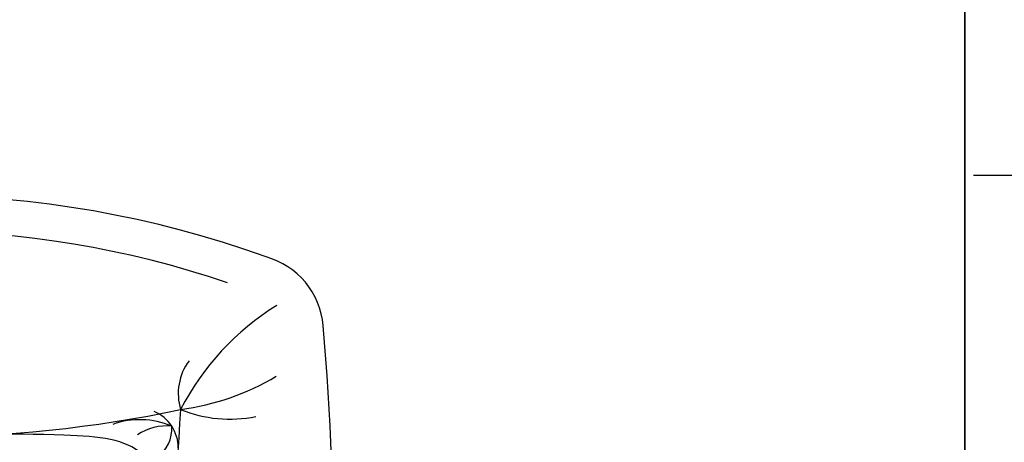
# Model space of a CAD drawing. Units: inches. Extents: x 844 to 2234, y 346 to 1084.
# Tile 88 of 93: x 2010.87 to 2030.9, y 728.83 to 737.43. Entities that reach past the tile are written whole.
import ezdxf

# ---------------------------------------------------------------- set-up
doc = ezdxf.new("R2010")
doc.units = ezdxf.units.IN
doc.header["$MEASUREMENT"] = 0
for name, color, linetype, lineweight in [('A-ANNO-DIMS', 2, 'Continuous', 18), ('A-WALL', 7, 'Continuous', 35), ('furniture', 8, 'Continuous', 18)]:
    doc.layers.add(name, color=color, linetype=linetype, lineweight=lineweight)
doc.layers.add('RA-AP-01$0$FURN', color=3, linetype='Continuous')
doc.layers.add('RA-AP-01$0$WOOD', color=64, linetype='Continuous')
doc.styles.get("Standard").update_dxf_attribs({"font": 'arial.ttf'})
doc.dimstyles.get("Standard").update_dxf_attribs({"dimtxt": 6, "dimasz": 3, "dimexe": 0.18, "dimexo": 0.0625, "dimgap": 0.09, "dimtad": 0, "dimtih": 1, "dimtoh": 1, "dimdec": 1, "dimzin": 0, "dimdsep": 46, "dimlunit": 3, "dimtxsty": 'Standard', "dimblk": 'ARCHTICK', "dimcen": 0.09, "dimadec": 0, "dimazin": 0, "dimtfac": 1, "dimtdec": 1, "dimtofl": 0, "dimtmove": 0, "dimatfit": 3, "dimfxl": 1, "dimtolj": 1, "dimtzin": 0, "dimarcsym": 0})

# ---------------------------------------------------------------- blocks, each defined once
blk = doc.blocks.new('A$C7F4351E2')
at = {"layer": 'RA-AP-01$0$FURN'}
for p, q in [((8.352559572600457, -8.263941955512525), (8.35255957259913, -8.282283310927069)), ((8.352559572600457, -8.927748273106442), (8.35255957259913, -8.909406917691898))]:
    blk.add_line(p, q, dxfattribs=at)
at = {"layer": 'RA-AP-01$0$FURN', "const_width": 0.01}
for points in [[(8.437812509519787, -8.415359762755768, 1), (8.427812509519786, -8.415359762755742, 1)], [(8.758197489244363, -8.415359762756214, -1), (8.768197489244365, -8.415359762756214, -1)], [(8.437812509519787, -8.776330465863198, -1), (8.427812509519786, -8.776330465863225, -1)], [(8.758197489244363, -8.776330465862753, 1), (8.768197489244365, -8.776330465862753, 1)]]:
    blk.add_lwpolyline(points, format="xyb", close=True, dxfattribs=at)
at = {"layer": 'RA-AP-01$0$FURN'}
for centre, radius, start, end in [((8.727559572604601, -11.61690445537682), 3.552808610866049, 85.0473312316413, 96.05887237565803), ((9.025650106946005, -8.176987401637472), 0.1, 15.499494600857, 85.04733123164159), ((8.50205957259015, -8.17394195551301), 0.1744999999876311, 148.9517780040467, 211.048221995953), ((8.77247054904813, -7.958543863781743), 0.3382138395168437, 297.2303327094027, 328.2563708342649), ((9.2484631175852, -8.302692737637487), 0.3241573581843151, 149.2985674842688, 172.3026350986055), ((7.88981694267423, -8.595845114309485), 1.310286319972027, 340.1192502251003, 19.8807497748998), ((9.084915705374858, -8.196040134964925), 0.1698955038956699, 168.877843135945, 201.8512383801196), ((7.929864357850293, -8.595845114309483), 1.224941341589781, 341.1257460634955, 18.87425393650447), ((8.947672844970796, -8.191835192646359), 0.0704710051510922, 253.1338634205325, 306.4126496157095), ((8.408522229993444, -8.33300072568355), 0.0753785023123622, 115.8745619060558, 163.9833547230034), ((8.603635103111959, -3.79706073025477), 4.473931917517753, 266.7828902523826, 274.1477233631118), ((8.878389979098333, -8.312202545234353), 0.05, 30.14777190425723, 89.99999999905349), ((10.52713941284929, -8.595845114309466), 1.634931324962266, 168.1200364254424, 191.8799635745573), ((9.101231010340802, -8.38034106221356), 0.5100538472773755, 167.6182489359307, 193.3122231353938), ((8.903279781571525, -8.31837865610295), 0.0478550828899777, 86.575295631534, 142.6833829238214), ((8.838100984994732, -8.276822957859652), 0.0683206773889159, 326.6729861493449, 5.218395042636973), ((8.810121490949696, -8.31110757721543), 0.1042084262671507, 340.4828318717155, 22.86929393278168), ((8.395364730619693, -8.304213854581548), 0.0479292786975047, 152.8070868543555, 225.4025460716553), ((8.333592787569726, -8.402663469525104), 0.1218651776285568, 48.0375529564433, 81.04623209541253), ((7.439612310514541, -8.913795367824825), 1.11020813118073, 31.93286085977143, 34.66647731879807), ((8.553131949433, -8.344109762755968), 0.1214118203512435, 150.1419074485596, 187.691663289156), ((8.642878049331348, -8.344109762756093), 0.1214118203512435, 352.3083367106845, 29.85809255128089), ((9.82633505008426, -8.696671375220811), 1.539060359583382, 165.5338783218257, 176.2437734318419), ((8.546954810732721, -8.753394424755975), 0.3517162425384579, 83.41248966761125, 103.1674570565571), ((8.697701155637269, -8.172468128267624), 0.2442261434243043, 248.9017070735605, 275.9923925191661), ((8.374918524725835, -8.294321202996931), 0.1212957045587361, 247.3375839744822, 273.7314750942433), ((8.73287643248165, -8.469775898206471), 0.3023568492824586, 173.0944825511667, 197.588060785551), ((8.889871101981017, -8.492307869305423), 0.1295083186917369, 167.9901339202812, 211.3796151021958), ((8.444145567704187, -7.829943385268752), 0.765467899454341, 258.6273206109321, 281.4174148186357), ((8.781211457338294, -7.772561243483908), 0.8232838708255751, 260.2449188973366, 277.7495311655964), ((9.82633505008426, -8.495018853398156), 1.539060359583382, 183.7562265681581, 194.4661216781742), ((8.444145567704187, -9.361312955433425), 0.765467899454341, 78.58258518136427, 101.3726793890678), ((8.781211457338294, -9.418695097218269), 0.8232838708255751, 82.25060502413102, 99.75508110266344), ((8.73287643248165, -8.721914330412496), 0.3023568492824586, 162.411939214449, 186.9055174488332), ((8.889871101981017, -8.699382359313544), 0.1295083186917369, 148.6203848978042, 192.0098660797188), ((9.101231010340802, -8.811349166405407), 0.5100538472773755, 166.6877768646062, 192.3817510640693), ((8.799643412436344, -8.749969313933361), 0.0689028341546707, 265.5384273543114, 353.5804828909086), ((8.374918524725835, -8.897369025622035), 0.1212957045587361, 86.26852490575668, 112.6624160255178), ((8.546954810732721, -8.438295803862992), 0.3517162425384579, 256.8325429434429, 276.5875103323888), ((8.697701155637269, -9.019222100351342), 0.2442261434243043, 84.00760748083387, 111.0982929264395), ((8.553131949433, -8.847580465862999), 0.1214118203512435, 172.308336710844, 209.8580925514404), ((8.785133372574222, -8.874256642962408), 0.0310151388417235, 42.62105484496073, 114.2239681486109), ((8.395364730619693, -8.88747637403742), 0.0479292786975047, 134.5974539283447, 207.1929131456445), ((8.810121490949696, -8.880582651403534), 0.1042084262671507, 337.1307060672183, 19.51716812828453), ((7.439612310514541, -8.277894860794142), 1.11020813118073, 325.333522681202, 328.0671391402286), ((8.408522229993444, -8.858689502935416), 0.0753785023123622, 196.0166452769965, 244.1254380939442), ((8.333592787569726, -8.789026759093863), 0.1218651776285568, 278.9537679045875, 311.9624470435567), ((8.838100984994732, -8.914867270759315), 0.0683206773889159, 354.781604957363, 33.32701385065517), ((8.642878049331348, -8.847580465862874), 0.1214118203512435, 330.1419074487191, 340.3913536181062), ((8.903279781571525, -8.873311572516016), 0.0478550828899777, 217.3166170761785, 273.424704368466), ((8.878389979098333, -8.879487683384612), 0.05, 270.0000000009465, 337.4173275753961), ((8.50205957259015, -9.017748273105955), 0.1744999999876311, 148.9517780040469, 211.0482219959533), ((8.603635103111959, -13.39462949836419), 4.473931917517753, 85.85227663688822, 93.21710974761734), ((9.084915705374858, -8.995650093654042), 0.1698955038956699, 158.1487616198804, 191.122156864055), ((8.947672844970796, -8.999855035972608), 0.0704710051510922, 53.58735038429053, 106.8661365794674), ((8.77247054904813, -9.233146364837223), 0.3382138395168437, 31.74362916573515, 62.76966729059727), ((9.2484631175852, -8.88899749098148), 0.3241573581843151, 187.6973649013944, 210.7014325157311), ((9.025650106946005, -9.014702826981493), 0.1, 274.9526687683584, 344.500505399143), ((8.727559572604601, -5.574785773242145), 3.552808610866049, 263.941127624342, 274.9526687683587)]:
    blk.add_arc(centre, radius, start, end, dxfattribs=at)
for points, knots in [([(8.764421239581775, -8.929562504990262), (8.755250524728652, -8.881106864374377), (8.74196437992213, -8.810906376383404), (8.80604948961138, -8.740469753734786), (8.847474678848357, -8.701097198289744), (8.897142214037096, -8.58322730303861), (8.897091569728207, -8.784804210134517), (8.88612504526093, -8.897825917224484), (8.806539053396843, -8.9185794820093), (8.764421239581775, -8.92956250499026)], [0, 0, 0, 0, 0.1367586589314792, 0.1981301758052368, 0.2677729570689282, 0.3281194902553322, 0.4737578340741565, 0.5765194025309516, 0.6920332287422236, 0.6920332287422236, 0.6920332287422236, 0.6920332287422236]), ([(8.764421239581775, -8.92956250499026), (8.782204778269502, -8.914603263160053), (8.821592007255505, -8.881471326160916), (8.86917941606436, -8.814322636989944), (8.867818990542759, -8.729338202119969), (8.881231406199264, -8.676770566934765), (8.888101821971249, -8.649843164808122)], [0, 0, 0, 0, 0.070018540671015, 0.1550780383534498, 0.2344491945777043, 0.3178048737568289, 0.3178048737568289, 0.3178048737568289, 0.3178048737568289])]:
    blk.add_open_spline(points, degree=3, knots=knots, dxfattribs=at)
blk = doc.blocks.new('A$C5D2F253E')
at = {"layer": 'RA-AP-01$0$WOOD', "xscale": -1, "rotation": 180}
blk.add_blockref('A$C7F4351E2', (-7.164808785335935, -7.45332973198748), dxfattribs=at)
blk = doc.blocks.new('_ArchTick')
at = {"color": 0, "linetype": 'ByBlock', "const_width": 0.15}
blk.add_lwpolyline([(-0.5, -0.5), (0.5, 0.5)], dxfattribs=at)
blk = doc.blocks.new('*D121')
at = {"layer": 'A-ANNO-DIMS', "color": 0, "lineweight": -2, "transparency": 16777216}
for p, q in [((2030.271987351997, 734.262611118704), (2040.245275089302, 734.262611118704)), ((2040.065275089302, 734.262611118704), (2040.065275089302, 704.6043509484256)), ((2040.065275089302, 668.557359536674), (2040.065275089302, 698.2156197069523)), ((2030.271987351997, 668.557359536674), (2040.245275089302, 668.557359536674))]:
    blk.add_line(p, q, dxfattribs=at)
at = {"layer": 'Defpoints', "color": 0, "transparency": 16777216}
for p in [(2030.209487351997, 734.262611118704), (2040.065275089302, 734.262611118704), (2030.209487351997, 668.557359536674)]:
    blk.add_point(p, dxfattribs=at)
at = {"layer": 'A-ANNO-DIMS', "color": 0, "lineweight": -2, "transparency": 16777216, "xscale": 3, "yscale": 3, "zscale": 3}
for p, rotation in [((2040.065275089302, 734.262611118704), 90), ((2040.065275089302, 668.557359536674), 270)]:
    blk.add_blockref('_ArchTick', p, dxfattribs=dict(at, rotation=rotation))
at = {"layer": 'A-ANNO-DIMS', "color": 0, "transparency": 16777216, "insert": (2040.065275089302, 701.4099853276883), "char_height": 6, "attachment_point": 5}
blk.add_mtext('\\A1;LOUNGE SET 5\'-5 1/2" TYP.', dxfattribs=at)

msp = doc.modelspace()

# ---------------------------------------------------------------- linework, layer by layer
at = {"layer": 'A-WALL'}
msp.add_line((2030.099168352677, 766.4551697629895), (2030.099168352677, 629.4551697629895), dxfattribs=at)

# ---------------------------------------------------------------- block references
at = {"layer": 'furniture', "xscale": -15.94108302203742, "yscale": 15.94108302203742, "zscale": 15.94108302203742, "rotation": 270}
msp.add_blockref('A$C5D2F253E', (1990.567271852805, 701.4028671565849), dxfattribs=at)

# ---------------------------------------------------------------- dimensions: what is measured, and where the dimension line sits
at = {"layer": 'A-ANNO-DIMS'}
dim = msp.add_linear_dim(base=(2040.065275089302, 734.262611118704), p1=(2030.209487351996, 668.5573595366737), p2=(2030.209487351996, 734.2626111187037), angle=90, text='LOUNGE SET <> TYP.', dimstyle='Standard', override={"dimdec": 1, "dimlfac": 1, "dimrnd": 0, "dimzin": 1, "dimdsep": 46, "dimlunit": 4, "dimfrac": 2}, dxfattribs=at)
dim.commit()
dim.dimension.update_dxf_attribs({"geometry": '*D121', "text_midpoint": (2040.065275089302, 701.4099853276883)})

doc.saveas('drawing.dxf')
